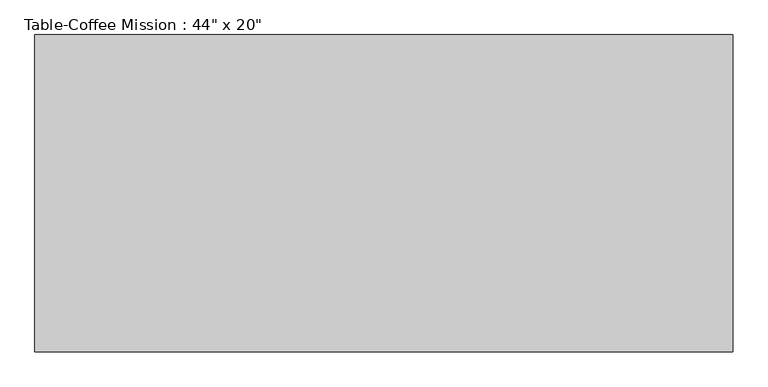
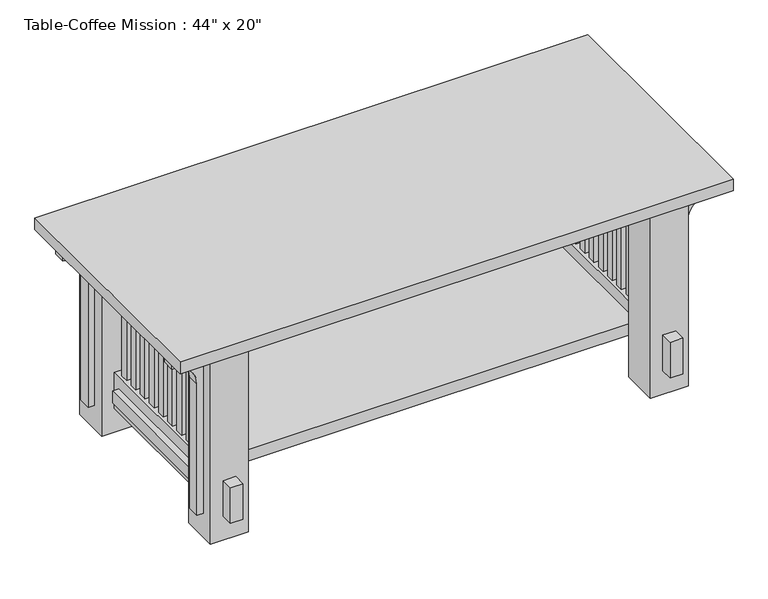
"""IFC4 building model written with IfcOpenShell, lengths in millimetres: furniture geometry."""

from ifc_helpers import new_model, si_unit, point, frame, frame_2d, origin, place, context, project, spatial, polyline, circle_curve, trimmed, segment, composite_curve, outline, extrude, faceted_brep, source, transform, mapped, element, save


def furniture_74675f9f(model_context):
    return source(origin(), model_context, "Body", "SolidModel", [
        extrude(outline(polyline([(558.8, 254.0), (558.8, -254.0), (-558.8, -254.0), (-558.8, 254.0), (558.8, 254.0)])), frame((0.0, 0.0, 406.4), z_axis=(0.0, 0.0, 1.0), x_axis=(1.0, 0.0, 0.0)), (0.0, 0.0, 1.0), 25.4),
        extrude(outline(polyline([(-438.15, 136.3578947), (-438.15, 120.3157895), (-450.85, 120.3157895), (-450.85, 136.3578947), (-438.15, 136.3578947)])), frame((0.0, 0.0, 127.0), z_axis=(0.0, 0.0, 1.0), x_axis=(1.0, 0.0, 0.0)), (0.0, 0.0, 1.0), 279.4),
        extrude(outline(polyline([(-438.15, -136.3578947), (-450.85, -136.3578947), (-450.85, -120.3157895), (-438.15, -120.3157895), (-438.15, -136.3578947)])), frame((0.0, 0.0, 127.0), z_axis=(0.0, 0.0, 1.0), x_axis=(1.0, 0.0, 0.0)), (0.0, 0.0, 1.0), 279.4),
        extrude(outline(polyline([(-438.15, -8.0210526), (-450.85, -8.0210526), (-450.85, 8.0210526), (-438.15, 8.0210526), (-438.15, -8.0210526)])), frame((0.0, 0.0, 127.0), z_axis=(0.0, 0.0, 1.0), x_axis=(1.0, 0.0, 0.0)), (0.0, 0.0, 1.0), 279.4),
        extrude(outline(polyline([(-438.15, 72.1894737), (-438.15, 56.1473684), (-450.85, 56.1473684), (-450.85, 72.1894737), (-438.15, 72.1894737)])), frame((0.0, 0.0, 127.0), z_axis=(0.0, 0.0, 1.0), x_axis=(1.0, 0.0, 0.0)), (0.0, 0.0, 1.0), 279.4),
        extrude(outline(polyline([(-438.15, -72.1894737), (-450.85, -72.1894737), (-450.85, -56.1473684), (-438.15, -56.1473684), (-438.15, -72.1894737)])), frame((0.0, 0.0, 127.0), z_axis=(0.0, 0.0, 1.0), x_axis=(1.0, 0.0, 0.0)), (0.0, 0.0, 1.0), 279.4),
        extrude(outline(polyline([(-438.15, -104.2736842), (-450.85, -104.2736842), (-450.85, -88.2315789), (-438.15, -88.2315789), (-438.15, -104.2736842)])), frame((0.0, 0.0, 127.0), z_axis=(0.0, 0.0, 1.0), x_axis=(1.0, 0.0, 0.0)), (0.0, 0.0, 1.0), 279.4),
        extrude(outline(polyline([(-438.15, -40.1052632), (-450.85, -40.1052632), (-450.85, -24.0631579), (-438.15, -24.0631579), (-438.15, -40.1052632)])), frame((0.0, 0.0, 127.0), z_axis=(0.0, 0.0, 1.0), x_axis=(1.0, 0.0, 0.0)), (0.0, 0.0, 1.0), 279.4),
        extrude(outline(polyline([(-438.15, 24.0631579), (-450.85, 24.0631579), (-450.85, 40.1052632), (-438.15, 40.1052632), (-438.15, 24.0631579)])), frame((0.0, 0.0, 127.0), z_axis=(0.0, 0.0, 1.0), x_axis=(1.0, 0.0, 0.0)), (0.0, 0.0, 1.0), 279.4),
        extrude(outline(polyline([(-438.15, 104.2736842), (-438.15, 88.2315789), (-450.85, 88.2315789), (-450.85, 104.2736842), (-438.15, 104.2736842)])), frame((0.0, 0.0, 127.0), z_axis=(0.0, 0.0, 1.0), x_axis=(1.0, 0.0, 0.0)), (0.0, 0.0, 1.0), 279.4),
        extrude(outline(polyline([(450.85, 136.3578947), (450.85, 120.3157895), (438.15, 120.3157895), (438.15, 136.3578947), (450.85, 136.3578947)])), frame((0.0, 0.0, 127.0), z_axis=(0.0, 0.0, 1.0), x_axis=(1.0, 0.0, 0.0)), (0.0, 0.0, 1.0), 279.4),
        extrude(outline(polyline([(450.85, 104.2736842), (450.85, 88.2315789), (438.15, 88.2315789), (438.15, 104.2736842), (450.85, 104.2736842)])), frame((0.0, 0.0, 127.0), z_axis=(0.0, 0.0, 1.0), x_axis=(1.0, 0.0, 0.0)), (0.0, 0.0, 1.0), 279.4),
        extrude(outline(polyline([(450.85, 72.1894737), (450.85, 56.1473684), (438.15, 56.1473684), (438.15, 72.1894737), (450.85, 72.1894737)])), frame((0.0, 0.0, 127.0), z_axis=(0.0, 0.0, 1.0), x_axis=(1.0, 0.0, 0.0)), (0.0, 0.0, 1.0), 279.4),
        extrude(outline(polyline([(450.85, 40.1052632), (450.85, 24.0631579), (438.15, 24.0631579), (438.15, 40.1052632), (450.85, 40.1052632)])), frame((0.0, 0.0, 127.0), z_axis=(0.0, 0.0, 1.0), x_axis=(1.0, 0.0, 0.0)), (0.0, 0.0, 1.0), 279.4),
        extrude(outline(polyline([(450.85, 8.0210526), (450.85, -8.0210526), (438.15, -8.0210526), (438.15, 8.0210526), (450.85, 8.0210526)])), frame((0.0, 0.0, 127.0), z_axis=(0.0, 0.0, 1.0), x_axis=(1.0, 0.0, 0.0)), (0.0, 0.0, 1.0), 279.4),
        extrude(outline(polyline([(450.85, -24.0631579), (450.85, -40.1052632), (438.15, -40.1052632), (438.15, -24.0631579), (450.85, -24.0631579)])), frame((0.0, 0.0, 127.0), z_axis=(0.0, 0.0, 1.0), x_axis=(1.0, 0.0, 0.0)), (0.0, 0.0, 1.0), 279.4),
        extrude(outline(polyline([(450.85, -56.1473684), (450.85, -72.1894737), (438.15, -72.1894737), (438.15, -56.1473684), (450.85, -56.1473684)])), frame((0.0, 0.0, 127.0), z_axis=(0.0, 0.0, 1.0), x_axis=(1.0, 0.0, 0.0)), (0.0, 0.0, 1.0), 279.4),
        extrude(outline(polyline([(450.85, -88.2315789), (450.85, -104.2736842), (438.15, -104.2736842), (438.15, -88.2315789), (450.85, -88.2315789)])), frame((0.0, 0.0, 127.0), z_axis=(0.0, 0.0, 1.0), x_axis=(1.0, 0.0, 0.0)), (0.0, 0.0, 1.0), 279.4),
        extrude(outline(polyline([(450.85, -120.3157895), (450.85, -136.3578947), (438.15, -136.3578947), (438.15, -120.3157895), (450.85, -120.3157895)])), frame((0.0, 0.0, 127.0), z_axis=(0.0, 0.0, 1.0), x_axis=(1.0, 0.0, 0.0)), (0.0, 0.0, 1.0), 279.4),
        extrude(outline(composite_curve([segment(trimmed(circle_curve(frame_2d((330.2, -546.1)), 50.8), [point((381.0, -546.1))], [point((330.2, -495.3))], True, "CARTESIAN"), True, "CONTINUOUS"), segment(polyline([(330.2, -495.3), (50.8, -495.3), (50.8, -482.6), (406.4, -482.6), (406.4, -546.1), (381.0, -546.1)]), True, "CONTINUOUS")], self_intersect=False)), frame((0.0, 177.8, 0.0), z_axis=(0.0, 1.0, 0.0), x_axis=(0.0, 0.0, 1.0)), (0.0, 0.0, 1.0), 25.4),
        extrude(outline(composite_curve([segment(trimmed(circle_curve(frame_2d((330.2, -546.1)), 50.8), [point((381.0, -546.1))], [point((330.2, -495.3))], True, "CARTESIAN"), True, "CONTINUOUS"), segment(polyline([(330.2, -495.3), (50.8, -495.3), (50.8, -482.6), (406.4, -482.6), (406.4, -546.1), (381.0, -546.1)]), True, "CONTINUOUS")], self_intersect=False)), frame((0.0, -203.2, 0.0), z_axis=(0.0, 1.0, 0.0), x_axis=(0.0, 0.0, 1.0)), (0.0, 0.0, 1.0), 25.4),
        extrude(outline(composite_curve([segment(polyline([(381.0, 546.1), (406.4, 546.1), (406.4, 482.6), (50.8, 482.6), (50.8, 495.3), (330.2, 495.3)]), True, "CONTINUOUS"), segment(trimmed(circle_curve(frame_2d((330.2, 546.1)), 50.8), [point((330.2, 495.3))], [point((381.0, 546.1))], True, "CARTESIAN"), True, "CONTINUOUS")], self_intersect=False)), frame((0.0, 177.8, 0.0), z_axis=(0.0, 1.0, 0.0), x_axis=(0.0, 0.0, 1.0)), (0.0, 0.0, 1.0), 25.4),
        extrude(outline(composite_curve([segment(polyline([(381.0, 546.1), (406.4, 546.1), (406.4, 482.6), (50.8, 482.6), (50.8, 495.3), (330.2, 495.3)]), True, "CONTINUOUS"), segment(trimmed(circle_curve(frame_2d((330.2, 546.1)), 50.8), [point((330.2, 495.3))], [point((381.0, 546.1))], True, "CARTESIAN"), True, "CONTINUOUS")], self_intersect=False)), frame((0.0, -203.2, 0.0), z_axis=(0.0, 1.0, 0.0), x_axis=(0.0, 0.0, 1.0)), (0.0, 0.0, 1.0), 25.4),
        faceted_brep([(482.6, 228.6, 406.4), (406.4, 228.6, 406.4), (406.4, 152.4, 406.4), (482.6, 152.4, 406.4), (482.6, 228.6, 0.0), (482.6, 152.4, 0.0), (406.4, 152.4, 0.0), (406.4, 228.6, 0.0), (457.2, 228.6, 127.0), (431.8, 228.6, 127.0), (431.8, 228.6, 50.8), (457.2, 228.6, 50.8), (431.8, 152.4, 127.0), (457.2, 152.4, 127.0), (457.2, 152.4, 50.8), (431.8, 152.4, 50.8), (431.8, -152.4, 127.0), (457.2, -152.4, 127.0), (457.2, 254.0, 127.0), (431.8, 254.0, 127.0), (431.8, -254.0, 127.0), (457.2, -254.0, 127.0), (457.2, -228.6, 127.0), (431.8, -228.6, 127.0), (457.2, -152.4, 50.8), (431.8, -152.4, 50.8), (457.2, -254.0, 50.8), (431.8, -254.0, 50.8), (431.8, -228.6, 50.8), (457.2, -228.6, 50.8), (431.8, 254.0, 50.8), (457.2, 254.0, 50.8), (457.2, -136.3578947, 101.6), (457.2, 136.3578947, 101.6), (457.2, 136.3578947, 76.2), (457.2, -136.3578947, 76.2), (431.8, 136.3578947, 101.6), (431.8, -136.3578947, 101.6), (431.8, -136.3578947, 76.2), (431.8, 136.3578947, 76.2), (482.6, -152.4, 406.4), (406.4, -152.4, 406.4), (406.4, -228.6, 406.4), (482.6, -228.6, 406.4), (482.6, -152.4, 0.0), (482.6, -228.6, 0.0), (406.4, -228.6, 0.0), (406.4, -152.4, 0.0), (-406.4, 228.6, 406.4), (-482.6, 228.6, 406.4), (-482.6, 152.4, 406.4), (-406.4, 152.4, 406.4), (-406.4, 228.6, 0.0), (-406.4, 152.4, 0.0), (-482.6, 152.4, 0.0), (-482.6, 228.6, 0.0), (-431.8, 228.6, 127.0), (-457.2, 228.6, 127.0), (-457.2, 228.6, 50.8), (-431.8, 228.6, 50.8), (-457.2, 152.4, 127.0), (-431.8, 152.4, 127.0), (-431.8, 152.4, 50.8), (-457.2, 152.4, 50.8), (-406.4, -152.4, 406.4), (-482.6, -152.4, 406.4), (-482.6, -228.6, 406.4), (-406.4, -228.6, 406.4), (-406.4, -152.4, 0.0), (-406.4, -228.6, 0.0), (-482.6, -228.6, 0.0), (-482.6, -152.4, 0.0), (-431.8, -152.4, 127.0), (-457.2, -152.4, 127.0), (-457.2, -152.4, 50.8), (-431.8, -152.4, 50.8), (-457.2, -228.6, 127.0), (-431.8, -228.6, 127.0), (-431.8, -228.6, 50.8), (-457.2, -228.6, 50.8), (-457.2, -254.0, 127.0), (-431.8, -254.0, 127.0), (-431.8, 254.0, 127.0), (-457.2, 254.0, 127.0), (-457.2, 254.0, 50.8), (-431.8, 254.0, 50.8), (-431.8, -254.0, 50.8), (-457.2, -254.0, 50.8), (-431.8, -136.3578947, 101.6), (-431.8, 136.3578947, 101.6), (-431.8, 136.3578947, 76.2), (-431.8, -136.3578947, 76.2), (-457.2, 136.3578947, 101.6), (-457.2, -136.3578947, 101.6), (-457.2, -136.3578947, 76.2), (-457.2, 136.3578947, 76.2), (-469.9, 136.3578947, 101.6), (-469.9, -136.3578947, 101.6), (469.9, -136.3578947, 101.6), (469.9, 136.3578947, 101.6), (469.9, 136.3578947, 76.2), (469.9, -136.3578947, 76.2), (-469.9, -136.3578947, 76.2), (-469.9, 136.3578947, 76.2)], [[[0, 1, 2, 3]], [[4, 5, 6, 7]], [[1, 0, 4, 7], [8, 9, 10, 11]], [[2, 1, 7, 6]], [[3, 2, 6, 5], [12, 13, 14, 15]], [[0, 3, 5, 4]], [[13, 12, 16, 17]], [[18, 19, 9, 8]], [[20, 21, 22, 23]], [[15, 14, 24, 25]], [[26, 27, 28, 29]], [[30, 31, 11, 10]], [[14, 13, 17, 24], [32, 33, 34, 35]], [[21, 26, 29, 22]], [[31, 18, 8, 11]], [[19, 18, 31, 30]], [[12, 15, 25, 16], [36, 37, 38, 39]], [[19, 30, 10, 9]], [[27, 20, 23, 28]], [[21, 20, 27, 26]], [[40, 41, 42, 43]], [[44, 45, 46, 47]], [[41, 40, 44, 47], [17, 16, 25, 24]], [[42, 41, 47, 46]], [[43, 42, 46, 45], [23, 22, 29, 28]], [[40, 43, 45, 44]], [[48, 49, 50, 51]], [[52, 53, 54, 55]], [[49, 48, 52, 55], [56, 57, 58, 59]], [[50, 49, 55, 54]], [[51, 50, 54, 53], [60, 61, 62, 63]], [[48, 51, 53, 52]], [[64, 65, 66, 67]], [[68, 69, 70, 71]], [[65, 64, 68, 71], [72, 73, 74, 75]], [[66, 65, 71, 70]], [[67, 66, 70, 69], [76, 77, 78, 79]], [[64, 67, 69, 68]], [[80, 81, 77, 76]], [[82, 83, 57, 56]], [[72, 61, 60, 73]], [[84, 85, 59, 58]], [[86, 87, 79, 78]], [[74, 63, 62, 75]], [[81, 80, 87, 86]], [[61, 72, 75, 62], [88, 89, 90, 91]], [[81, 86, 78, 77]], [[85, 82, 56, 59]], [[83, 82, 85, 84]], [[73, 60, 63, 74], [92, 93, 94, 95]], [[87, 80, 76, 79]], [[83, 84, 58, 57]], [[96, 97, 93, 92]], [[98, 99, 33, 32]], [[36, 89, 88, 37]], [[100, 101, 35, 34]], [[102, 103, 95, 94]], [[38, 91, 90, 39]], [[89, 36, 39, 90]], [[99, 100, 34, 33]], [[103, 96, 92, 95]], [[97, 96, 103, 102]], [[37, 88, 91, 38]], [[97, 102, 94, 93]], [[101, 98, 32, 35]], [[99, 98, 101, 100]]]),
    ])


if __name__ == "__main__":
    model = new_model("IFC4")
    model_context = context("Model", 3, world=origin())
    ifc_project = project(units=[si_unit("LENGTHUNIT", "METRE", prefix="MILLI")], contexts=[model_context])
    site = spatial("IfcSite", under=ifc_project)
    building = spatial("IfcBuilding", under=site)
    placement = place(None, origin())
    furniture_shape = furniture_74675f9f(model_context)
    element("IfcFurniture", 1, ObjectType="Table-Coffee Mission : 44\" x 20\"", at=placement, inside=building, context=model_context, shape_type="MappedRepresentation", body=[
        mapped(furniture_shape, transform((0.0, 0.0, 0.0), x_axis=(1.0, 0.0, 0.0), y_axis=(0.0, 1.0, 0.0), z_axis=(0.0, 0.0, 1.0))),
    ])
    save(model, "model.ifc")

# Revit data of these elements
# Type "Table-Coffee Mission : 44\" x 20\""
#   Assembly Code = "E2020200"
#   Height = 1' - 5"
#   Length = 3' - 8"
#   Width = 1' - 8"
#   Material = Wood - Mahogany
#   Default Elevation = 0
# Element 1 (IfcFurniture, "Table-Coffee Mission : 44\" x 20\"")
#   Materials on its faces: "Wood - Mahogany"
# Materials
#   "Wood - Mahogany": colour RGB 138 86 45, transparency 0
